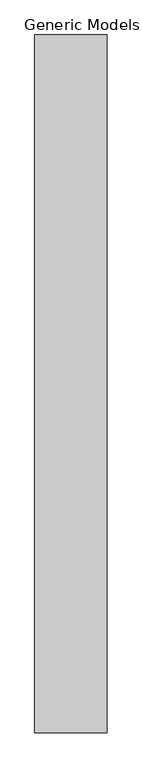
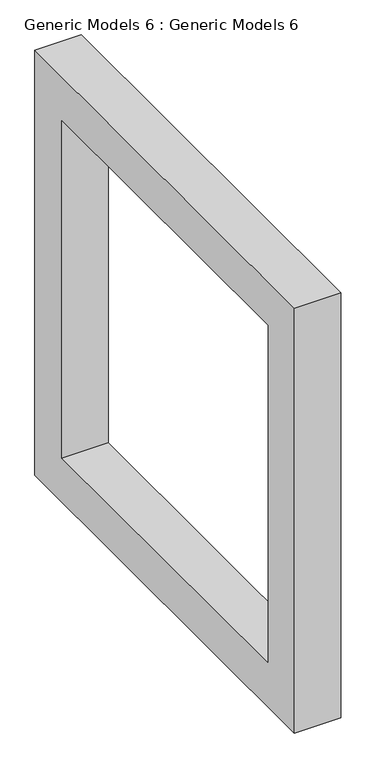
"""IFC4 building model written with IfcOpenShell, lengths in millimetres: proxy geometry, Generic Models 6 : Generic Models 6."""

from ifc_helpers import new_model, si_unit, frame, origin, place, context, project, spatial, polyline, outline, extrude, source, transform, mapped, element, save


def generic_models_6_generic_models_6_ceaf88ca(model_context):
    return source(origin(), model_context, "Body", "SweptSolid", [
        extrude(outline(polyline([(888.1500137, 5918.2), (888.1500137, 4445.0), (-585.0499863, 4445.0), (-585.0499863, 5918.2), (888.1500137, 5918.2)]), holes=[polyline([(735.7500137, 5765.8), (-432.6499863, 5765.8), (-432.6499863, 4597.4), (735.7500137, 4597.4), (735.7500137, 5765.8)])]), frame((-4753.1023867, 0.0, 0.0), z_axis=(1.0, 0.0, 0.0), x_axis=(0.0, 1.0, 0.0)), (0.0, 0.0, 1.0), 152.4),
    ])


if __name__ == "__main__":
    model = new_model("IFC4")
    model_context = context("Model", 3, world=origin())
    ifc_project = project(units=[si_unit("LENGTHUNIT", "METRE", prefix="MILLI")], contexts=[model_context])
    site = spatial("IfcSite", under=ifc_project)
    building = spatial("IfcBuilding", under=site)
    placement = place(None, origin())
    generic_models_6_generic_models_6_shape = generic_models_6_generic_models_6_ceaf88ca(model_context)
    element("IfcBuildingElementProxy", 1, Name="Generic Models 6 : Generic Models 6", ObjectType="Generic Models 6 : Generic Models 6", at=placement, inside=building, context=model_context, shape_type="MappedRepresentation", body=[
        mapped(generic_models_6_generic_models_6_shape, transform((0.0, 0.0, 0.0), x_axis=(1.0, 0.0, 0.0), y_axis=(0.0, 1.0, 0.0), z_axis=(0.0, 0.0, 1.0))),
    ])
    save(model, "model.ifc")

# Revit data of these elements
# Element 1 (IfcBuildingElementProxy, "Generic Models 6 : Generic Models 6")
#   Materials on its faces: "accent wall"
# Materials
#   "accent wall": class "Generic", colour RGB 120 120 120, transparency 0, Cost = 0
